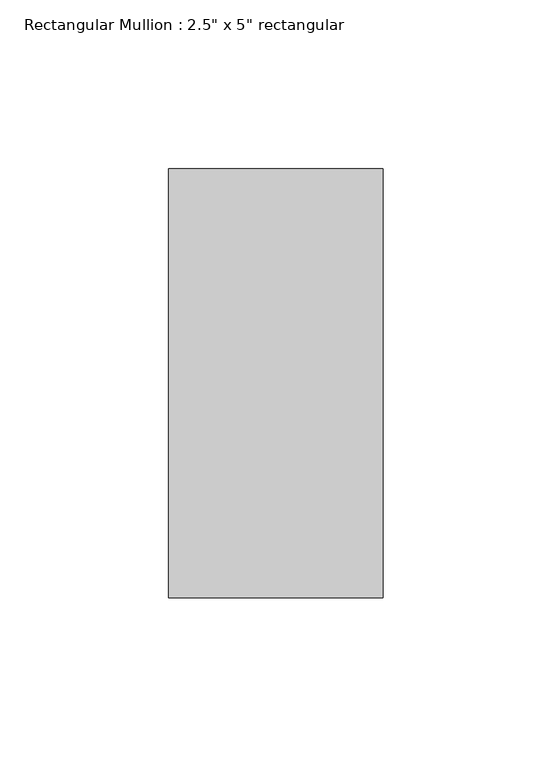
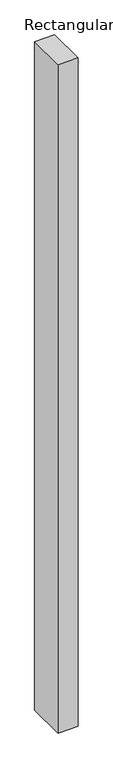
"""IFC4 building model written with IfcOpenShell, lengths in millimetres: member geometry."""

from ifc_helpers import new_model, si_unit, frame, origin, place, context, project, spatial, polyline, outline, extrude, source, transform, mapped, element, save


def member_5f9244a4(model_context):
    return source(origin(), model_context, "Body", "SweptSolid", [
        extrude(outline(polyline([(0.0, 63.5), (0.0, -63.5), (-63.5, -63.5), (-63.5, 63.5), (0.0, 63.5)])), frame((0.0, 0.0, -2234.5154028), z_axis=(0.0, 0.0, 1.0), x_axis=(1.0, 0.0, 0.0)), (0.0, 0.0, 1.0), 2234.5154028),
    ])


if __name__ == "__main__":
    model = new_model("IFC4")
    model_context = context("Model", 3, world=origin())
    ifc_project = project(units=[si_unit("LENGTHUNIT", "METRE", prefix="MILLI")], contexts=[model_context])
    site = spatial("IfcSite", under=ifc_project)
    building = spatial("IfcBuilding", under=site)
    placement = place(None, origin())
    member_shape = member_5f9244a4(model_context)
    element("IfcMember", 1, ObjectType="Rectangular Mullion : 2.5\" x 5\" rectangular", at=placement, inside=building, context=model_context, shape_type="MappedRepresentation", body=[
        mapped(member_shape, transform((0.0, 0.0, 0.0), x_axis=(1.0, 0.0, 0.0), y_axis=(0.0, 1.0, 0.0), z_axis=(0.0, 0.0, 1.0))),
    ])
    save(model, "model.ifc")

# Revit data of these elements
# Type "Rectangular Mullion : 2.5\" x 5\" rectangular"
#   built-in parameter 1007304 = 0.416667 (stored number, unit not read)
#   built-in parameter 1007301 = 0.104167 (stored number, unit not read)
#   built-in parameter 1007300 = 0.104167 (stored number, unit not read)
# Element 1 (IfcMember, "Rectangular Mullion : 2.5\" x 5\" rectangular")
#   Materials on its faces: "Aluminum"
# Materials
#   "Aluminum": class "Metal", colour RGB 247 247 247, transparency 0, Description = "Aluminum 6061", Cost = 0
